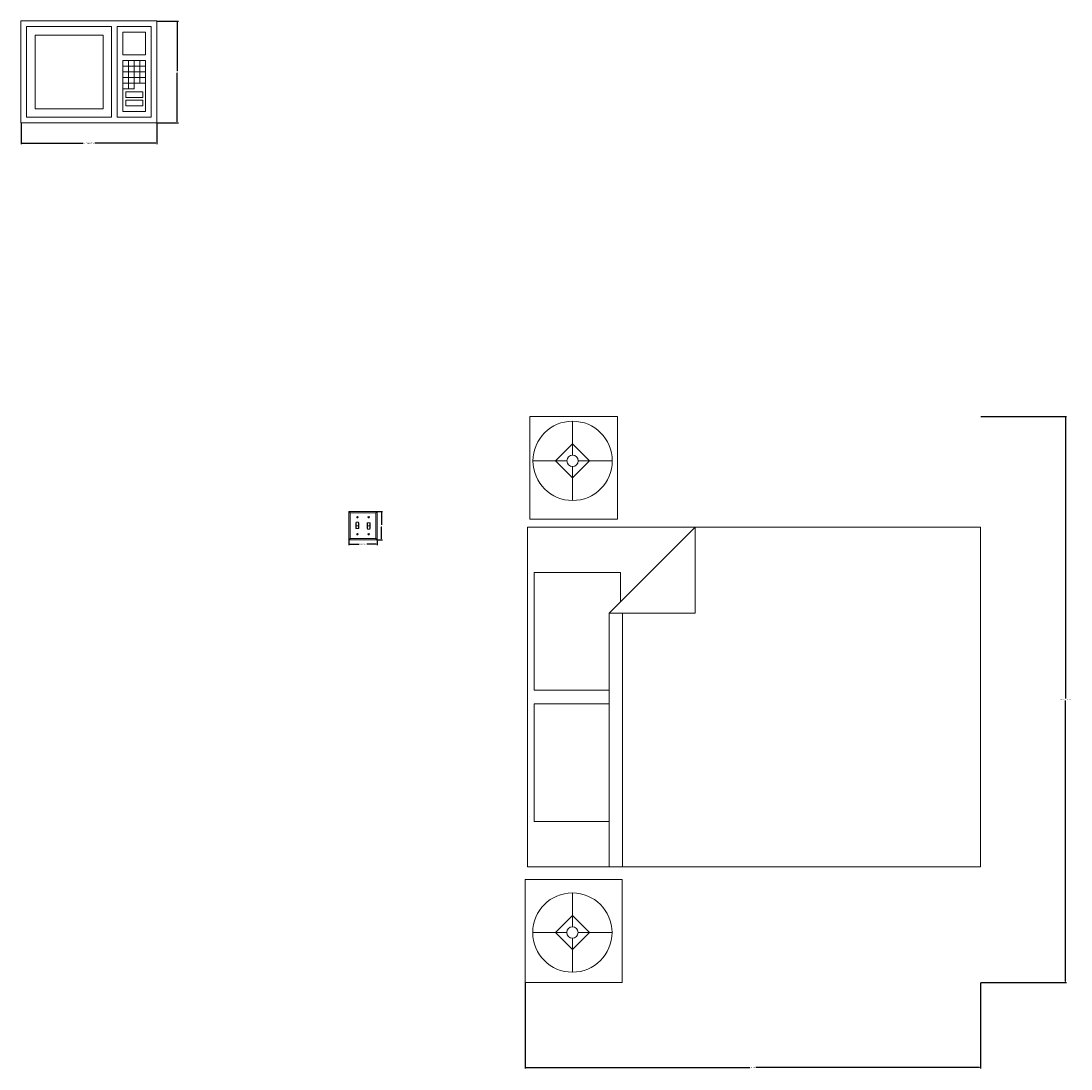
# Model space of a CAD drawing. Units: inches. Extents: x -52 to 1967, y 32 to 824.
# Tile 9 of 10: x 1580 to 1766, y 479 to 664. Entities that reach past the tile are written whole.
import ezdxf

# ---------------------------------------------------------------- set-up
doc = ezdxf.new("R2010")
doc.units = ezdxf.units.IN
for name, color, linetype, lineweight in [('A-ANNO-DIMS', 2, 'Continuous', 18), ('A-EQPM', 9, 'Continuous', 18), ('A-FURN', 8, 'Continuous', 18), ('E-LITE', 2, 'Continuous', 18)]:
    doc.layers.add(name, color=color, linetype=linetype, lineweight=lineweight)
doc.styles.get("Standard").update_dxf_attribs({"font": 'arial.ttf'})
doc.dimstyles.get("Standard").update_dxf_attribs({"dimtxt": 0.18, "dimasz": 0.18, "dimexe": 0.18, "dimexo": 0.0625, "dimgap": 0.09, "dimtad": 0, "dimtih": 1, "dimtoh": 1, "dimdec": 4, "dimzin": 0, "dimdsep": 46, "dimtxsty": 'Standard', "dimcen": 0.09, "dimadec": 0, "dimazin": 0, "dimtfac": 1, "dimtdec": 4, "dimtofl": 0, "dimtmove": 0, "dimatfit": 3, "dimfxl": 1, "dimtolj": 1, "dimtzin": 0, "dimarcsym": 0})

# ---------------------------------------------------------------- blocks, each defined once
blk = doc.blocks.new('Light Switch - Dual')
for p, q in [((-2.25, 4.75), (-2.5, 5)), ((-2.25, 4.75), (2.25, 4.75)), ((-2.25, 0.25), (-2.25, 4.75)), ((-0.875, 4), (-1.125, 4)), ((0.875, 4), (1.125, 4)), ((2.25, 4.75), (2.5, 5)), ((2.25, 4.75), (2.25, 0.25)), ((-0.7854, 2.5), (-1.2183, 2.5)), ((0.7854, 2.5), (1.2182, 2.5)), ((-2.25, 0.25), (-2.5, 0)), ((2.25, 0.25), (-2.25, 0.25)), ((-0.875, 1), (-1.125, 1)), ((0.875, 1), (1.125, 1)), ((2.25, 0.25), (2.5, 0))]:
    blk.add_line(p, q)
for points in [[(-2.5, 0), (-2.5, 5), (2.5, 5), (2.5, 0)], [(-0.78, 3.125), (-0.78, 2), (-1.22, 2), (-1.22, 3.125)], [(0.78, 1.875), (0.78, 3), (1.22, 3), (1.22, 1.875)]]:
    blk.add_lwpolyline(points, close=True)
for points in [[(-0.7818, 3), (-0.75, 3), (-0.75, 2), (-1.25, 2), (-1.25, 3), (-1.2219, 3)], [(0.7817, 2), (0.75, 2), (0.75, 3), (1.25, 3), (1.25, 2), (1.2219, 2)]]:
    blk.add_lwpolyline(points)
for centre in [(-1, 4), (1, 4), (-1, 1), (1, 1)]:
    blk.add_circle(centre, 0.125)
blk = doc.blocks.new('Microwave')
for p, q in [((18, 10), (22, 10)), ((19, 7), (19, 11)), ((20, 11), (20, 7)), ((21, 7), (21, 11)), ((22, 9), (18, 9)), ((18, 8), (22, 8)), ((22, 7), (18, 7)), ((20, 6), (18, 6)), ((19, 6), (19, 7)), ((20, 7), (20, 6))]:
    blk.add_line(p, q)
for points in [[(0, 0), (0, 18), (24, 18), (24, 0)], [(1, 1), (1, 17), (16, 17), (16, 1)], [(17, 1), (17, 17), (23, 17), (23, 1)], [(2.5, 2.5), (2.5, 15.5), (14.5, 15.5), (14.5, 2.5)], [(18, 12), (18, 16), (22, 16), (22, 12)], [(18, 2), (18, 11), (22, 11), (22, 2)], [(18.5, 4.5), (18.5, 5.5), (21.5, 5.5), (21.5, 4.5)], [(18.5, 3), (18.5, 4), (21.5, 4), (21.5, 3)]]:
    blk.add_lwpolyline(points, close=True)
blk = doc.blocks.new('Bed - Queen')
for p, q in [((0, -80.00003), (0, 0)), ((0, 0), (59.99999, 0)), ((59.99999, 0), (59.99999, -80.00003)), ((7.99999, -1.2), (28.79998, -1.2)), ((7.99999, -14.4), (7.99999, -1.2)), ((28.79998, -1.2), (28.79998, -14.4)), ((31.19999, -1.2), (51.99999, -1.2)), ((31.19999, -14.4), (31.19999, -1.2)), ((51.99999, -1.2), (51.99999, -16.4)), ((0, -14.4), (44.8, -14.4)), ((59.99999, -29.6), (44.8, -14.4)), ((44.8, -14.4), (44.8, -29.6)), ((51.99999, -16.4), (46.79936, -16.4)), ((44.8, -16.8), (0, -16.8)), ((44.8, -29.6), (59.99999, -29.6)), ((59.99999, -80.00003), (0, -80.00003))]:
    blk.add_line(p, q)
blk = doc.blocks.new('Lamp - Table')
for p, q in [((0, 7), (0, 1)), ((0, 3), (-3, 0)), ((3, 0), (0, 3)), ((-1, 0), (-7, 0)), ((-3, 0), (0, -3)), ((0, -3), (3, 0)), ((1, 0), (7, 0)), ((0, -1), (0, -7))]:
    blk.add_line(p, q)
for radius in [7, 1]:
    blk.add_circle((0, 0), radius)
blk = doc.blocks.new('BED-QUEEN-WITH-NIGHTSTANDS')
for points in [[(0.4, 61.39), (15.92, 61.39), (15.92, 79.53), (0.4, 79.53)], [(-0.42, -2.26), (16.73, -2.26), (16.73, -20.45), (-0.42, -20.45)]]:
    blk.add_lwpolyline(points, close=True)
for p in [(7.97, 71.69), (7.93, -11.61)]:
    blk.add_blockref('Lamp - Table', p)
at = {"rotation": 90}
blk.add_blockref('Bed - Queen', (0, 0), dxfattribs=at)
blk = doc.blocks.new('*D27')
at = {"layer": 'A-ANNO-DIMS', "color": 0, "lineweight": -2, "transparency": 16777216}
for p, q in [((1749.73, 594.26), (1764.85, 594.26)), ((1764.67, 594.08), (1764.67, 544.45)), ((1764.67, 494.46), (1764.67, 544.08)), ((1749.73, 494.28), (1764.85, 494.28))]:
    blk.add_line(p, q, dxfattribs=at)
at = {"layer": 'A-ANNO-DIMS', "color": 0, "transparency": 16777216}
for points in [[(1764.64, 594.08), (1764.7, 594.08), (1764.67, 594.26)], [(1764.64, 494.46), (1764.7, 494.46), (1764.67, 494.28)]]:
    blk.add_solid(points, dxfattribs=at)
at = {"layer": 'Defpoints', "color": 0, "transparency": 16777216}
for p in [(1749.67, 594.26), (1764.67, 594.26), (1749.67, 494.28)]:
    blk.add_point(p, dxfattribs=at)
at = {"layer": 'A-ANNO-DIMS', "color": 0, "transparency": 16777216, "insert": (1764.67, 544.27), "char_height": 0.18, "attachment_point": 5}
blk.add_mtext('\\A1;BED SET 100 TYP.', dxfattribs=at)
blk = doc.blocks.new('*D28')
at = {"layer": 'A-ANNO-DIMS', "color": 0, "lineweight": -2, "transparency": 16777216}
for p, q in [((1669.25, 494.21), (1669.25, 479.1)), ((1749.67, 494.21), (1749.67, 479.1)), ((1669.43, 479.28), (1708.93, 479.28)), ((1749.49, 479.28), (1709.99, 479.28))]:
    blk.add_line(p, q, dxfattribs=at)
at = {"layer": 'A-ANNO-DIMS', "color": 0, "transparency": 16777216}
for points in [[(1669.43, 479.31), (1669.43, 479.25), (1669.25, 479.28)], [(1749.49, 479.31), (1749.49, 479.25), (1749.67, 479.28)]]:
    blk.add_solid(points, dxfattribs=at)
at = {"layer": 'Defpoints', "color": 0, "transparency": 16777216}
for p in [(1669.25, 494.28), (1749.67, 494.28), (1749.67, 479.28)]:
    blk.add_point(p, dxfattribs=at)
at = {"layer": 'A-ANNO-DIMS', "color": 0, "transparency": 16777216, "insert": (1709.46, 479.28), "char_height": 0.18, "attachment_point": 5}
blk.add_mtext('\\A1;80 TYP.', dxfattribs=at)
blk = doc.blocks.new('*D49')
at = {"layer": 'A-ANNO-DIMS', "color": 0, "lineweight": -2, "transparency": 16777216}
for p, q in [((1580.24, 646.03), (1580.24, 642.31)), ((1604.24, 646.03), (1604.24, 642.31)), ((1580.42, 642.49), (1591.2, 642.49)), ((1604.06, 642.49), (1593.28, 642.49))]:
    blk.add_line(p, q, dxfattribs=at)
at = {"layer": 'A-ANNO-DIMS', "color": 0, "transparency": 16777216}
for points in [[(1580.42, 642.52), (1580.42, 642.46), (1580.24, 642.49)], [(1604.06, 642.52), (1604.06, 642.46), (1604.24, 642.49)]]:
    blk.add_solid(points, dxfattribs=at)
at = {"layer": 'Defpoints', "color": 0, "transparency": 16777216}
for p in [(1580.24, 646.09), (1604.24, 646.09), (1604.24, 642.49)]:
    blk.add_point(p, dxfattribs=at)
at = {"layer": 'A-ANNO-DIMS', "color": 0, "transparency": 16777216, "insert": (1592.24, 642.49), "char_height": 0.18, "attachment_point": 5}
blk.add_mtext('\\A1;MICROWAVE 24', dxfattribs=at)
blk = doc.blocks.new('*D50')
at = {"layer": 'A-ANNO-DIMS', "color": 0, "lineweight": -2, "transparency": 16777216}
for p, q in [((1604.3, 664.09), (1608.02, 664.09)), ((1607.84, 663.91), (1607.84, 655.27)), ((1607.84, 646.27), (1607.84, 654.91)), ((1604.3, 646.09), (1608.02, 646.09))]:
    blk.add_line(p, q, dxfattribs=at)
at = {"layer": 'A-ANNO-DIMS', "color": 0, "transparency": 16777216}
for points in [[(1607.81, 663.91), (1607.87, 663.91), (1607.84, 664.09)], [(1607.81, 646.27), (1607.87, 646.27), (1607.84, 646.09)]]:
    blk.add_solid(points, dxfattribs=at)
at = {"layer": 'Defpoints', "color": 0, "transparency": 16777216}
for p in [(1604.24, 664.09), (1607.84, 664.09), (1604.24, 646.09)]:
    blk.add_point(p, dxfattribs=at)
at = {"layer": 'A-ANNO-DIMS', "color": 0, "transparency": 16777216, "insert": (1607.84, 655.09), "char_height": 0.18, "attachment_point": 5}
blk.add_mtext('\\A1;18', dxfattribs=at)
blk = doc.blocks.new('*D51')
at = {"layer": 'A-ANNO-DIMS', "color": 0, "lineweight": -2, "transparency": 16777216}
for p, q in [((1638.13, 572.39), (1638.13, 571.52)), ((1638.31, 571.7), (1639.95, 571.7)), ((1642.95, 571.7), (1641.31, 571.7)), ((1643.13, 572.39), (1643.13, 571.52))]:
    blk.add_line(p, q, dxfattribs=at)
at = {"layer": 'A-ANNO-DIMS', "color": 0, "transparency": 16777216}
for points in [[(1638.31, 571.73), (1638.31, 571.67), (1638.13, 571.7)], [(1642.95, 571.73), (1642.95, 571.67), (1643.13, 571.7)]]:
    blk.add_solid(points, dxfattribs=at)
at = {"layer": 'Defpoints', "color": 0, "transparency": 16777216}
for p in [(1638.13, 572.45), (1643.13, 572.45), (1643.13, 571.7)]:
    blk.add_point(p, dxfattribs=at)
at = {"layer": 'A-ANNO-DIMS', "color": 0, "transparency": 16777216, "insert": (1640.63, 571.7), "char_height": 0.18, "attachment_point": 5}
blk.add_mtext('\\A1;SWITCH 5', dxfattribs=at)
blk = doc.blocks.new('*D52')
at = {"layer": 'A-ANNO-DIMS', "color": 0, "lineweight": -2, "transparency": 16777216}
for p, q in [((1643.2, 577.45), (1644.06, 577.45)), ((1643.88, 577.27), (1643.88, 575.14)), ((1643.88, 572.63), (1643.88, 574.77)), ((1643.2, 572.45), (1644.06, 572.45))]:
    blk.add_line(p, q, dxfattribs=at)
at = {"layer": 'A-ANNO-DIMS', "color": 0, "transparency": 16777216}
for points in [[(1643.85, 577.27), (1643.91, 577.27), (1643.88, 577.45)], [(1643.85, 572.63), (1643.91, 572.63), (1643.88, 572.45)]]:
    blk.add_solid(points, dxfattribs=at)
at = {"layer": 'Defpoints', "color": 0, "transparency": 16777216}
for p in [(1643.13, 577.45), (1643.88, 577.45), (1643.13, 572.45)]:
    blk.add_point(p, dxfattribs=at)
at = {"layer": 'A-ANNO-DIMS', "color": 0, "transparency": 16777216, "insert": (1643.88, 574.95), "char_height": 0.18, "attachment_point": 5}
blk.add_mtext('\\A1;5', dxfattribs=at)

msp = doc.modelspace()

# ---------------------------------------------------------------- block references
at = {"layer": 'A-EQPM'}
msp.add_blockref('Microwave', (1580.2385, 646.0915), dxfattribs=at)
at = {"layer": 'A-FURN'}
msp.add_blockref('BED-QUEEN-WITH-NIGHTSTANDS', (1669.6682, 514.723), dxfattribs=at)
at = {"layer": 'E-LITE'}
msp.add_blockref('Light Switch - Dual', (1640.6344, 572.4549), dxfattribs=at)

# ---------------------------------------------------------------- dimensions: what is measured, and where the dimension line sits
at = {"layer": 'A-ANNO-DIMS'}
for base, p1, p2, picture, middle in [((1607.8385, 664.0915), (1604.2385, 646.0915), (1604.2385, 664.0915), '*D50', (1607.8385, 655.0915)), ((1643.8844, 577.4549), (1643.1344, 572.4549), (1643.1344, 577.4549), '*D52', (1643.8844, 574.9549))]:
    dim = msp.add_linear_dim(base=base, p1=p1, p2=p2, angle=90, dimstyle='Standard', override={"dimdec": 0, "dimlfac": 1, "dimrnd": 0, "dimzin": 0, "dimdsep": 46, "dimlunit": 2}, dxfattribs=at)
    dim.commit()
    dim.dimension.update_dxf_attribs({"geometry": picture, "text_midpoint": middle})
for base, p1, p2, text, picture, middle in [((1604.2385, 642.4915), (1580.2385, 646.0915), (1604.2385, 646.0915), 'MICROWAVE <>', '*D49', (1592.2385, 642.4915)), ((1643.1344, 571.7049), (1638.1344, 572.4549), (1643.1344, 572.4549), 'SWITCH <>', '*D51', (1640.6344, 571.7049)), ((1749.6683, 479.2796), (1669.2466, 494.2765), (1749.6683, 494.2765), '<> TYP.', '*D28', (1709.4574, 479.2796))]:
    dim = msp.add_linear_dim(base=base, p1=p1, p2=p2, text=text, dimstyle='Standard', override={"dimdec": 0, "dimlfac": 1, "dimrnd": 0, "dimzin": 0, "dimdsep": 46, "dimlunit": 2}, dxfattribs=at)
    dim.commit()
    dim.dimension.update_dxf_attribs({"geometry": picture, "text_midpoint": middle})
dim = msp.add_linear_dim(base=(1764.6652, 594.2561), p1=(1749.6683, 494.2765), p2=(1749.6683, 594.2561), angle=90, text='BED SET <> TYP.', dimstyle='Standard', override={"dimdec": 0, "dimlfac": 1, "dimrnd": 0, "dimzin": 0, "dimdsep": 46, "dimlunit": 2}, dxfattribs=at)
dim.commit()
dim.dimension.update_dxf_attribs({"geometry": '*D27', "text_midpoint": (1764.6652, 544.2663)})

doc.saveas('drawing.dxf')
